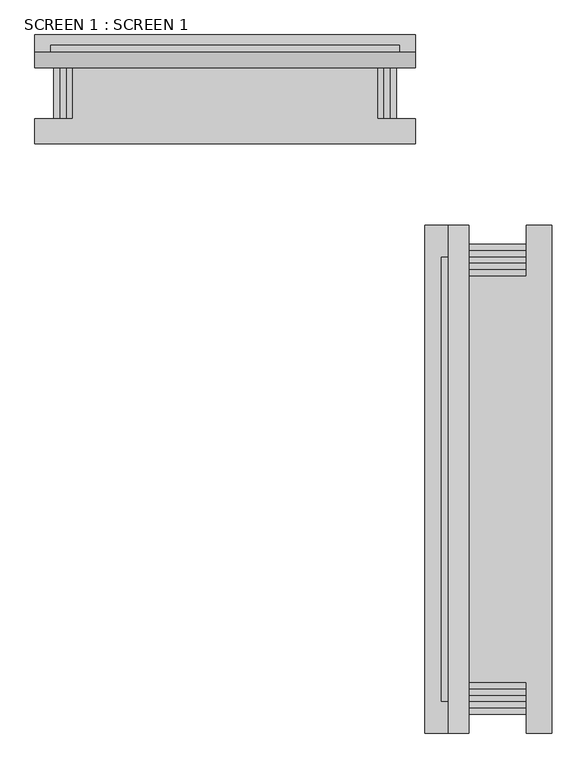
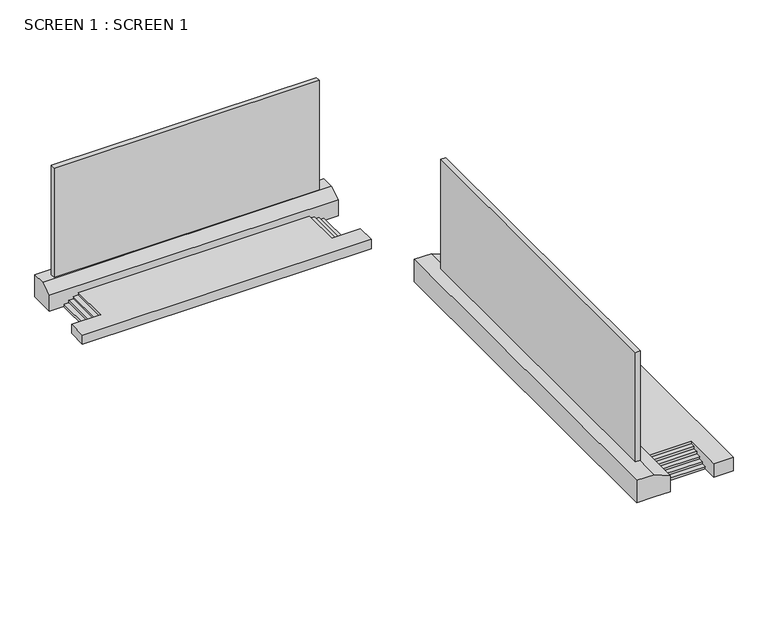
"""IFC4 building model written with IfcOpenShell, lengths in millimetres: proxy geometry, SCREEN 1 : SCREEN 1."""

from ifc_helpers import new_model, si_unit, point, frame, frame_2d, origin, origin_with_axes, place, context, project, spatial, polyline, circle_curve, trimmed, segment, composite_curve, outline, extrude, source, transform, mapped, element, save


def screen_1_screen_1_327eb079(model_context):
    return source(origin(), model_context, "Body", "SweptSolid", [
        extrude(outline(polyline([(346.6587563, 3880.8794445), (346.6587563, 1442.4794445), (41.8587563, 1442.4794445), (41.8587563, 3880.8794445), (346.6587563, 3880.8794445)])), origin_with_axes(), (0.0, 0.0, 1.0), 152.4),
        extrude(outline(polyline([(-16112.5412437, 3880.8794445), (-15807.7412437, 3880.8794445), (-15807.7412437, 1442.4794445), (-16112.5412437, 1442.4794445), (-16112.5412437, 3880.8794445)])), origin_with_axes(), (0.0, 0.0, 1.0), 152.4),
        extrude(outline(polyline([(41.8587563, 3880.8794445), (41.8587563, 1442.4794445), (-262.9412437, 1442.4794445), (-262.9412437, 3880.8794445), (41.8587563, 3880.8794445)])), origin_with_axes(), (0.0, 0.0, 1.0), 304.8),
        extrude(outline(polyline([(-15807.7412437, 3880.8794445), (-15502.9412437, 3880.8794445), (-15502.9412437, 1442.4794445), (-15807.7412437, 1442.4794445), (-15807.7412437, 3880.8794445)])), origin_with_axes(), (0.0, 0.0, 1.0), 304.8),
        extrude(outline(polyline([(-262.9412437, 3880.8794445), (-262.9412437, 1442.4794445), (-567.7412437, 1442.4794445), (-567.7412437, 3880.8794445), (-262.9412437, 3880.8794445)])), origin_with_axes(), (0.0, 0.0, 1.0), 457.2),
        extrude(outline(polyline([(-15502.9412437, 3880.8794445), (-15198.1412437, 3880.8794445), (-15198.1412437, 1442.4794445), (-15502.9412437, 1442.4794445), (-15502.9412437, 3880.8794445)])), origin_with_axes(), (0.0, 0.0, 1.0), 457.2),
        extrude(outline(polyline([(-15198.1412437, 3880.8794445), (-567.7412437, 3880.8794445), (-567.7412437, 1442.4794445), (1261.0587563, 1442.4794445), (1261.0587563, 251.561128), (-17026.9412437, 251.561128), (-17026.9412437, 1442.4794445), (-15198.1412437, 1442.4794445), (-15198.1412437, 3880.8794445)])), origin_with_axes(), (0.0, 0.0, 1.0), 609.6),
        extrude(outline(polyline([(6582.3587563, -4894.8205555), (3839.1587563, -4894.8205555), (3839.1587563, -4590.0205555), (6582.3587563, -4590.0205555), (6582.3587563, -4894.8205555)])), origin_with_axes(), (0.0, 0.0, 1.0), 152.4),
        extrude(outline(polyline([(6582.3587563, -26840.4205555), (6582.3587563, -27145.2205555), (3839.1587563, -27145.2205555), (3839.1587563, -26840.4205555), (6582.3587563, -26840.4205555)])), origin_with_axes(), (0.0, 0.0, 1.0), 152.4),
        extrude(outline(polyline([(6582.3587563, -5199.6205555), (3839.1587563, -5199.6205555), (3839.1587563, -4894.8205555), (6582.3587563, -4894.8205555), (6582.3587563, -5199.6205555)])), origin_with_axes(), (0.0, 0.0, 1.0), 304.8),
        extrude(outline(polyline([(6582.3587563, -26535.6205555), (6582.3587563, -26840.4205555), (3839.1587563, -26840.4205555), (3839.1587563, -26535.6205555), (6582.3587563, -26535.6205555)])), origin_with_axes(), (0.0, 0.0, 1.0), 304.8),
        extrude(outline(polyline([(6582.3587563, -5504.4205555), (3839.1587563, -5504.4205555), (3839.1587563, -5199.6205555), (6582.3587563, -5199.6205555), (6582.3587563, -5504.4205555)])), origin_with_axes(), (0.0, 0.0, 1.0), 457.2),
        extrude(outline(polyline([(6582.3587563, -26230.8205555), (6582.3587563, -26535.6205555), (3839.1587563, -26535.6205555), (3839.1587563, -26230.8205555), (6582.3587563, -26230.8205555)])), origin_with_axes(), (0.0, 0.0, 1.0), 457.2),
        extrude(outline(polyline([(6582.3587563, -5809.2205555), (3839.1587563, -5809.2205555), (3839.1587563, -5504.4205555), (6582.3587563, -5504.4205555), (6582.3587563, -5809.2205555)])), origin_with_axes(), (0.0, 0.0, 1.0), 609.6),
        extrude(outline(polyline([(6582.3587563, -25926.0205555), (6582.3587563, -26230.8205555), (3839.1587563, -26230.8205555), (3839.1587563, -25926.0205555), (6582.3587563, -25926.0205555)])), origin_with_axes(), (0.0, 0.0, 1.0), 609.6),
        extrude(outline(polyline([(6582.3587563, -6114.0205555), (3839.1587563, -6114.0205555), (3839.1587563, -5809.2205555), (6582.3587563, -5809.2205555), (6582.3587563, -6114.0205555)])), origin_with_axes(), (0.0, 0.0, 1.0), 762.0),
        extrude(outline(polyline([(6582.3587563, -25621.2205555), (6582.3587563, -25926.0205555), (3839.1587563, -25926.0205555), (3839.1587563, -25621.2205555), (6582.3587563, -25621.2205555)])), origin_with_axes(), (0.0, 0.0, 1.0), 762.0),
        extrude(outline(polyline([(7821.7393908, -3675.6205555), (7821.7393908, -28059.6205555), (6582.3587563, -28059.6205555), (6582.3587563, -25621.2205555), (3839.1587563, -25621.2205555), (3839.1587563, -6114.0205555), (6582.3587563, -6114.0205555), (6582.3587563, -3675.6205555), (7821.7393908, -3675.6205555)])), origin_with_axes(), (0.0, 0.0, 1.0), 914.4),
        extrude(outline(polyline([(5468.3794445, 1498.6), (5468.3794445, 0.0), (4642.8794445, 0.0), (3880.8794445, 0.0), (3880.8794445, 1066.8), (4630.1794445, 1498.6), (5468.3794445, 1498.6)])), frame((-17026.9412437, 0.0, 0.0), z_axis=(1.0, 0.0, 0.0), x_axis=(0.0, 1.0, 0.0)), (0.0, 0.0, 1.0), 18288.0),
        extrude(outline(polyline([(1490.3196, 1718.2587563), (0.0, 1718.2587563), (0.0, 2823.1587563), (0.0, 3839.1587563), (1066.8, 3839.1587563), (1490.3196, 2823.1587563), (1490.3196, 1718.2587563)])), frame((0.0, -28059.6205555, 0.0), z_axis=(0.0, 1.0, 0.0), x_axis=(0.0, 0.0, 1.0)), (0.0, 0.0, 1.0), 24384.0),
        extrude(outline(composite_curve([segment(trimmed(circle_curve(frame_2d((-7882.9412437, -116900.1902636)), 121857.0915096), [point((499.0587563, 4668.2794445))], [point((-16264.9412437, 4668.2794445))], True, "CARTESIAN"), True, "CONTINUOUS"), segment(polyline([(-16264.9412437, 4668.2794445), (-16264.9412437, 4973.8012736)]), True, "CONTINUOUS"), segment(trimmed(circle_curve(frame_2d((-7882.9412437, -116900.1902636)), 122161.8915096), [point((-16264.9412437, 4973.8012736))], [point((499.0587563, 4973.8012736))], False, "CARTESIAN"), True, "CONTINUOUS"), segment(polyline([(499.0587563, 4973.8012736), (499.0587563, 4668.2794445)]), True, "CONTINUOUS")], self_intersect=False)), frame((0.0, 0.0, 1524.0), z_axis=(0.0, 0.0, 1.0), x_axis=(1.0, 0.0, 0.0)), (0.0, 0.0, 1.0), 7315.2),
        extrude(outline(composite_curve([segment(trimmed(circle_curve(frame_2d((122185.1541652, -15867.6205555)), 119837.7743953), [point((2823.1587563, -5199.6205555))], [point((2823.1587563, -26535.6205555))], True, "CARTESIAN"), True, "CONTINUOUS"), segment(polyline([(2823.1587563, -26535.6205555), (2517.1469188, -26535.6205555)]), True, "CONTINUOUS"), segment(trimmed(circle_curve(frame_2d((122185.1541652, -15867.6205555)), 120142.5743953), [point((2517.1469188, -26535.6205555))], [point((2517.1469188, -5199.6205555))], False, "CARTESIAN"), True, "CONTINUOUS"), segment(polyline([(2517.1469188, -5199.6205555), (2823.1587563, -5199.6205555)]), True, "CONTINUOUS")], self_intersect=False)), frame((0.0, 0.0, 1524.0), z_axis=(0.0, 0.0, 1.0), x_axis=(1.0, 0.0, 0.0)), (0.0, 0.0, 1.0), 7315.2),
    ])


if __name__ == "__main__":
    model = new_model("IFC4")
    model_context = context("Model", 3, world=origin())
    ifc_project = project(units=[si_unit("LENGTHUNIT", "METRE", prefix="MILLI")], contexts=[model_context])
    site = spatial("IfcSite", under=ifc_project)
    building = spatial("IfcBuilding", under=site)
    placement = place(None, origin())
    screen_1_screen_1_shape = screen_1_screen_1_327eb079(model_context)
    element("IfcBuildingElementProxy", 1, Name="SCREEN 1 : SCREEN 1", ObjectType="SCREEN 1 : SCREEN 1", at=placement, inside=building, context=model_context, shape_type="MappedRepresentation", body=[
        mapped(screen_1_screen_1_shape, transform((0.0, 0.0, 0.0), x_axis=(1.0, 0.0, 0.0), y_axis=(0.0, 1.0, 0.0), z_axis=(0.0, 0.0, 1.0))),
    ])
    save(model, "model.ifc")
